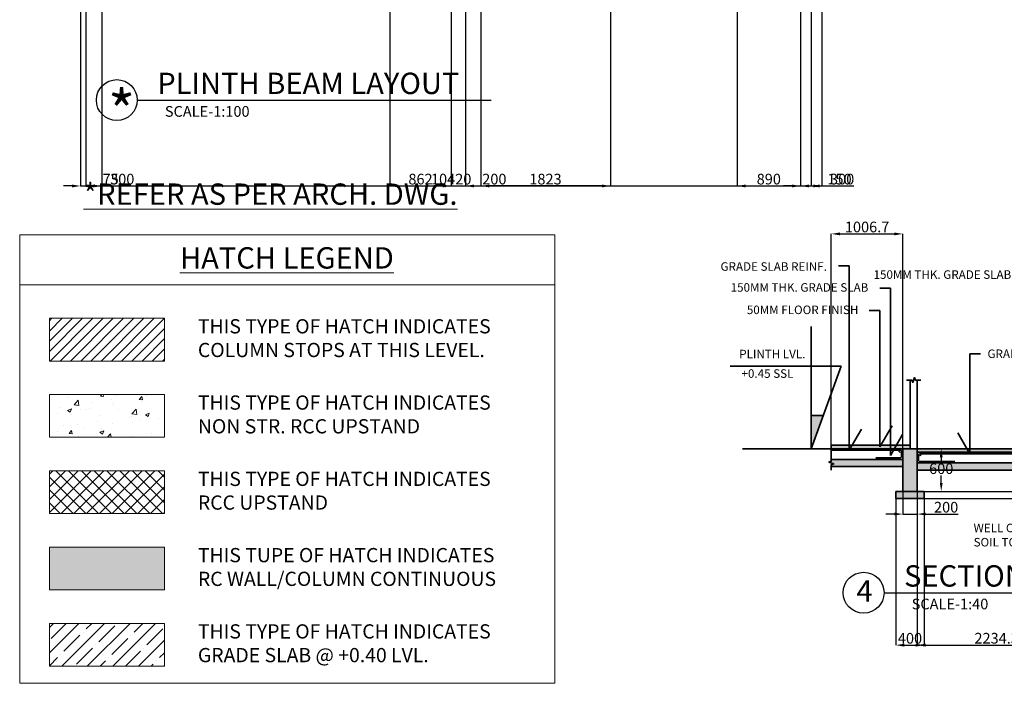
# Model space of a CAD drawing. Units: millimetres. Extents: x -174 to 32373, y 27344 to 53129.
# Tile 2 of 7: x 7596 to 21438, y 27344 to 36674. Entities that reach past the tile are written whole.
import ezdxf

# ---------------------------------------------------------------- set-up
doc = ezdxf.new("R2010")
doc.units = ezdxf.units.MM
doc.header["$LTSCALE"] = 50
for name, color, linetype, lineweight in [('S-ANNO-DIMS', 2, 'Continuous', 18), ('S-ANNO-LEGD', 7, 'Continuous', 18), ('S-ANNO-SYMB', 4, 'Continuous', 25), ('S-ANNO-TEXT', 3, 'Continuous', 18), ('S-DETL', 7, 'Continuous', 35), ('S-PATT', 8, 'Continuous', 13), ('S-REIN', 1, 'Continuous', 25)]:
    doc.layers.add(name, color=color, linetype=linetype, lineweight=lineweight)
doc.styles.get("Standard").update_dxf_attribs({"font": 'arial.ttf'})
doc.dimstyles.new('ISO-25', dxfattribs={"dimtxt": 150, "dimasz": 120, "dimexe": 1.25, "dimexo": 0.625, "dimtad": 1, "dimtih": 1, "dimtoh": 1, "dimdec": 0, "dimtxsty": 'Standard', "dimcen": 2.5, "dimadec": 0, "dimazin": 0, "dimtfac": 1, "dimtdec": 0, "dimtmove": 0, "dimatfit": 3, "dimfxl": 1, "dimarcsym": 0})

# ---------------------------------------------------------------- blocks, each defined once
blk = doc.blocks.new('*D26')
at = {"layer": 'Defpoints', "color": 0, "transparency": 16777216}
for p in [(20012, 30042), (20212, 30042), (20212, 29723)]:
    blk.add_point(p, dxfattribs=at)
at = {"layer": 'S-ANNO-DIMS', "color": 0, "lineweight": -2, "transparency": 16777216}
for p, q in [((20012, 30041), (20012, 29722)), ((20212, 30041), (20212, 29722)), ((19892, 29723), (19772, 29723)), ((20012, 29723), (20212, 29723)), ((20332, 29723), (20787, 29723))]:
    blk.add_line(p, q, dxfattribs=at)
at = {"layer": 'S-ANNO-DIMS', "color": 0, "transparency": 16777216}
for points in [[(19892, 29743), (19892, 29703), (20012, 29723)], [(20332, 29743), (20332, 29703), (20212, 29723)]]:
    blk.add_solid(points, dxfattribs=at)
at = {"layer": 'S-ANNO-DIMS', "color": 0, "transparency": 16777216, "insert": (20620, 29800), "char_height": 150, "attachment_point": 5}
blk.add_mtext('200', dxfattribs=at)
blk = doc.blocks.new('*D28')
at = {"layer": 'Defpoints', "color": 0, "transparency": 16777216}
for p in [(20212, 30642), (20212, 30042), (20551, 30042)]:
    blk.add_point(p, dxfattribs=at)
at = {"layer": 'S-ANNO-DIMS', "color": 0, "lineweight": -2, "transparency": 16777216}
for p, q in [((20213, 30642), (20552, 30642)), ((20551, 30522), (20551, 30419)), ((20551, 30162), (20551, 30265)), ((20213, 30042), (20552, 30042))]:
    blk.add_line(p, q, dxfattribs=at)
at = {"layer": 'S-ANNO-DIMS', "color": 0, "transparency": 16777216}
for points in [[(20531, 30522), (20571, 30522), (20551, 30642)], [(20531, 30162), (20571, 30162), (20551, 30042)]]:
    blk.add_solid(points, dxfattribs=at)
at = {"layer": 'S-ANNO-DIMS', "color": 0, "transparency": 16777216, "insert": (20551, 30342), "char_height": 150, "attachment_point": 5}
blk.add_mtext('600', dxfattribs=at)
blk = doc.blocks.new('SECTION-MARK')
blk.add_line((575, 287), (4248, 287))
blk.add_circle((287, 287), 287)
blk = doc.blocks.new('*D36')
at = {"layer": 'Defpoints', "color": 0, "transparency": 16777216}
for p in [(8452, 38444), (18872, 38369), (18872, 34336)]:
    blk.add_point(p, dxfattribs=at)
at = {"layer": 'S-ANNO-DIMS', "color": 0, "lineweight": -2, "transparency": 16777216}
for p, q in [((8452, 38443), (8452, 34335)), ((18872, 38368), (18872, 34335)), ((8572, 34336), (18752, 34336))]:
    blk.add_line(p, q, dxfattribs=at)
at = {"layer": 'S-ANNO-DIMS', "color": 0, "transparency": 16777216}
for points in [[(8572, 34356), (8572, 34316), (8452, 34336)], [(18752, 34356), (18752, 34316), (18872, 34336)]]:
    blk.add_solid(points, dxfattribs=at)
at = {"layer": 'S-ANNO-DIMS', "color": 0, "transparency": 16777216, "insert": (13662, 34413), "char_height": 150, "attachment_point": 5}
blk.add_mtext('10420', dxfattribs=at)
blk = doc.blocks.new('*D37')
at = {"layer": 'Defpoints', "color": 0, "transparency": 16777216}
for p in [(8452, 38444), (8527, 36932), (8527, 34336)]:
    blk.add_point(p, dxfattribs=at)
at = {"layer": 'S-ANNO-DIMS', "color": 0, "lineweight": -2, "transparency": 16777216}
for p, q in [((8452, 38443), (8452, 34335)), ((8527, 36931), (8527, 34335)), ((8332, 34336), (8212, 34336)), ((8452, 34336), (8527, 34336)), ((8647, 34336), (8983, 34336))]:
    blk.add_line(p, q, dxfattribs=at)
at = {"layer": 'S-ANNO-DIMS', "color": 0, "transparency": 16777216}
for points in [[(8332, 34356), (8332, 34316), (8452, 34336)], [(8647, 34356), (8647, 34316), (8527, 34336)]]:
    blk.add_solid(points, dxfattribs=at)
at = {"layer": 'S-ANNO-DIMS', "color": 0, "transparency": 16777216, "insert": (8875, 34413), "char_height": 150, "attachment_point": 5}
blk.add_mtext('75', dxfattribs=at)
blk = doc.blocks.new('*D38')
at = {"layer": 'Defpoints', "color": 0, "transparency": 16777216}
for p in [(18572, 38369), (18722, 36932), (18722, 34336)]:
    blk.add_point(p, dxfattribs=at)
at = {"layer": 'S-ANNO-DIMS', "color": 0, "lineweight": -2, "transparency": 16777216}
for p, q in [((18572, 38368), (18572, 34335)), ((18722, 36931), (18722, 34335)), ((18452, 34336), (18332, 34336)), ((18572, 34336), (18722, 34336)), ((18842, 34336), (19280, 34336))]:
    blk.add_line(p, q, dxfattribs=at)
at = {"layer": 'S-ANNO-DIMS', "color": 0, "transparency": 16777216}
for points in [[(18452, 34356), (18452, 34316), (18572, 34336)], [(18842, 34356), (18842, 34316), (18722, 34336)]]:
    blk.add_solid(points, dxfattribs=at)
at = {"layer": 'S-ANNO-DIMS', "color": 0, "transparency": 16777216, "insert": (19121, 34413), "char_height": 150, "attachment_point": 5}
blk.add_mtext('150', dxfattribs=at)
blk = doc.blocks.new('*D41')
at = {"layer": 'Defpoints', "color": 0, "transparency": 16777216}
for p in [(8452, 38444), (8752, 38444), (8752, 34336)]:
    blk.add_point(p, dxfattribs=at)
at = {"layer": 'S-ANNO-DIMS', "color": 0, "lineweight": -2, "transparency": 16777216}
for p, q in [((8452, 38443), (8452, 34335)), ((8752, 38443), (8752, 34335)), ((8572, 34336), (8632, 34336)), ((8752, 34336), (9204, 34336))]:
    blk.add_line(p, q, dxfattribs=at)
at = {"layer": 'S-ANNO-DIMS', "color": 0, "transparency": 16777216}
for points in [[(8572, 34356), (8572, 34316), (8452, 34336)], [(8632, 34356), (8632, 34316), (8752, 34336)]]:
    blk.add_solid(points, dxfattribs=at)
at = {"layer": 'S-ANNO-DIMS', "color": 0, "transparency": 16777216, "insert": (9038, 34413), "char_height": 150, "attachment_point": 5}
blk.add_mtext('300', dxfattribs=at)
blk = doc.blocks.new('*D44')
at = {"layer": 'Defpoints', "color": 0, "transparency": 16777216}
for p in [(13662, 45234), (13862, 45234), (13862, 34336)]:
    blk.add_point(p, dxfattribs=at)
at = {"layer": 'S-ANNO-DIMS', "color": 0, "lineweight": -2, "transparency": 16777216}
for p, q in [((13662, 45233), (13662, 34335)), ((13862, 45233), (13862, 34335)), ((13542, 34336), (13422, 34336)), ((13662, 34336), (13862, 34336)), ((13982, 34336), (14436, 34336))]:
    blk.add_line(p, q, dxfattribs=at)
at = {"layer": 'S-ANNO-DIMS', "color": 0, "transparency": 16777216}
for points in [[(13542, 34356), (13542, 34316), (13662, 34336)], [(13982, 34356), (13982, 34316), (13862, 34336)]]:
    blk.add_solid(points, dxfattribs=at)
at = {"layer": 'S-ANNO-DIMS', "color": 0, "transparency": 16777216, "insert": (14269, 34413), "char_height": 150, "attachment_point": 5}
blk.add_mtext('200', dxfattribs=at)
blk = doc.blocks.new('*D46')
at = {"layer": 'Defpoints', "color": 0, "transparency": 16777216}
for p in [(18572, 38369), (18872, 38369), (18872, 34336)]:
    blk.add_point(p, dxfattribs=at)
at = {"layer": 'S-ANNO-DIMS', "color": 0, "lineweight": -2, "transparency": 16777216}
for p, q in [((18572, 38368), (18572, 34335)), ((18872, 38368), (18872, 34335)), ((18692, 34336), (18752, 34336)), ((18872, 34336), (19324, 34336))]:
    blk.add_line(p, q, dxfattribs=at)
at = {"layer": 'S-ANNO-DIMS', "color": 0, "transparency": 16777216}
for points in [[(18692, 34356), (18692, 34316), (18572, 34336)], [(18752, 34356), (18752, 34316), (18872, 34336)]]:
    blk.add_solid(points, dxfattribs=at)
at = {"layer": 'S-ANNO-DIMS', "color": 0, "transparency": 16777216, "insert": (19158, 34413), "char_height": 150, "attachment_point": 5}
blk.add_mtext('300', dxfattribs=at)
blk = doc.blocks.new('*D48')
at = {"layer": 'Defpoints', "color": 0, "transparency": 16777216}
for p in [(17682, 43024), (18572, 38669), (18572, 34336)]:
    blk.add_point(p, dxfattribs=at)
at = {"layer": 'S-ANNO-DIMS', "color": 0, "lineweight": -2, "transparency": 16777216}
for p, q in [((17682, 43023), (17682, 34335)), ((18572, 38668), (18572, 34335)), ((17802, 34336), (18452, 34336))]:
    blk.add_line(p, q, dxfattribs=at)
at = {"layer": 'S-ANNO-DIMS', "color": 0, "transparency": 16777216}
for points in [[(17802, 34356), (17802, 34316), (17682, 34336)], [(18452, 34356), (18452, 34316), (18572, 34336)]]:
    blk.add_solid(points, dxfattribs=at)
at = {"layer": 'S-ANNO-DIMS', "color": 0, "transparency": 16777216, "insert": (18127, 34413), "char_height": 150, "attachment_point": 5}
blk.add_mtext('890', dxfattribs=at)
blk = doc.blocks.new('*D58')
at = {"layer": 'Defpoints', "color": 0, "transparency": 16777216}
for p in [(15900, 43174), (14077, 43024), (14077, 34336)]:
    blk.add_point(p, dxfattribs=at)
at = {"layer": 'S-ANNO-DIMS', "color": 0, "lineweight": -2, "transparency": 16777216}
for p, q in [((15900, 43173), (15900, 34335)), ((14077, 43023), (14077, 34335)), ((15780, 34336), (14197, 34336))]:
    blk.add_line(p, q, dxfattribs=at)
at = {"layer": 'S-ANNO-DIMS', "color": 0, "transparency": 16777216}
for points in [[(14197, 34356), (14197, 34316), (14077, 34336)], [(15780, 34356), (15780, 34316), (15900, 34336)]]:
    blk.add_solid(points, dxfattribs=at)
at = {"layer": 'S-ANNO-DIMS', "color": 0, "transparency": 16777216, "insert": (14988, 34413), "char_height": 150, "attachment_point": 5}
blk.add_mtext('1823', dxfattribs=at)
blk = doc.blocks.new('*D59')
at = {"layer": 'Defpoints', "color": 0, "transparency": 16777216}
for p in [(12800, 46609), (13662, 46609), (13662, 34336)]:
    blk.add_point(p, dxfattribs=at)
at = {"layer": 'S-ANNO-DIMS', "color": 0, "lineweight": -2, "transparency": 16777216}
for p, q in [((12800, 46608), (12800, 34335)), ((13662, 46608), (13662, 34335)), ((12920, 34336), (13542, 34336))]:
    blk.add_line(p, q, dxfattribs=at)
at = {"layer": 'S-ANNO-DIMS', "color": 0, "transparency": 16777216}
for points in [[(12920, 34356), (12920, 34316), (12800, 34336)], [(13542, 34356), (13542, 34316), (13662, 34336)]]:
    blk.add_solid(points, dxfattribs=at)
at = {"layer": 'S-ANNO-DIMS', "color": 0, "transparency": 16777216, "insert": (13231, 34413), "char_height": 150, "attachment_point": 5}
blk.add_mtext('862', dxfattribs=at)
blk = doc.blocks.new('*D85')
at = {"layer": 'Defpoints', "color": 0, "transparency": 16777216}
for p in [(20212, 30042), (22447, 30042), (22447, 27880)]:
    blk.add_point(p, dxfattribs=at)
at = {"layer": 'S-ANNO-DIMS', "color": 0, "lineweight": -2, "transparency": 16777216}
for p, q in [((20212, 30041), (20212, 27879)), ((22447, 30041), (22447, 27879)), ((20332, 27880), (22327, 27880))]:
    blk.add_line(p, q, dxfattribs=at)
at = {"layer": 'S-ANNO-DIMS', "color": 0, "transparency": 16777216}
for points in [[(20332, 27900), (20332, 27860), (20212, 27880)], [(22327, 27900), (22327, 27860), (22447, 27880)]]:
    blk.add_solid(points, dxfattribs=at)
at = {"layer": 'S-ANNO-DIMS', "color": 0, "transparency": 16777216, "insert": (21330, 27958), "char_height": 150, "attachment_point": 5}
blk.add_mtext('2234.3', dxfattribs=at)
blk = doc.blocks.new('*D89')
at = {"layer": 'Defpoints', "color": 0, "transparency": 16777216}
for p in [(20012, 33662), (19006, 30692), (20012, 30642)]:
    blk.add_point(p, dxfattribs=at)
at = {"layer": 'S-ANNO-DIMS', "color": 0, "lineweight": -2, "transparency": 16777216}
for p, q in [((19006, 30692), (19006, 33664)), ((19126, 33662), (19892, 33662)), ((20012, 30642), (20012, 33664))]:
    blk.add_line(p, q, dxfattribs=at)
at = {"layer": 'S-ANNO-DIMS', "color": 0, "transparency": 16777216}
for points in [[(19126, 33682), (19126, 33642), (19006, 33662)], [(19892, 33682), (19892, 33642), (20012, 33662)]]:
    blk.add_solid(points, dxfattribs=at)
at = {"layer": 'S-ANNO-DIMS', "color": 0, "transparency": 16777216, "insert": (19509, 33740), "char_height": 150, "attachment_point": 5}
blk.add_mtext('1006.7', dxfattribs=at)
blk = doc.blocks.new('*D91')
at = {"layer": 'Defpoints', "color": 0, "transparency": 16777216}
for p in [(19912, 29942), (20312, 29942), (20312, 27880)]:
    blk.add_point(p, dxfattribs=at)
at = {"layer": 'S-ANNO-DIMS', "color": 0, "lineweight": -2, "transparency": 16777216}
for p, q in [((19912, 29941), (19912, 27879)), ((20312, 29941), (20312, 27879)), ((20032, 27880), (20192, 27880))]:
    blk.add_line(p, q, dxfattribs=at)
at = {"layer": 'S-ANNO-DIMS', "color": 0, "transparency": 16777216}
for points in [[(20032, 27900), (20032, 27860), (19912, 27880)], [(20192, 27900), (20192, 27860), (20312, 27880)]]:
    blk.add_solid(points, dxfattribs=at)
at = {"layer": 'S-ANNO-DIMS', "color": 0, "transparency": 16777216, "insert": (20112, 27957), "char_height": 150, "attachment_point": 5}
blk.add_mtext('400', dxfattribs=at)
blk = doc.blocks.new('*D92')
at = {"layer": 'Defpoints', "color": 0, "transparency": 16777216}
for p in [(20312, 30042), (24149, 30042), (20312, 29942)]:
    blk.add_point(p, dxfattribs=at)
at = {"layer": 'S-ANNO-DIMS', "color": 0, "lineweight": -2, "transparency": 16777216}
for p, q in [((24149, 30162), (24149, 30282)), ((24149, 30282), (24466, 30282)), ((20313, 30042), (24150, 30042)), ((24149, 29942), (24149, 30042)), ((20313, 29942), (24150, 29942)), ((24149, 29822), (24149, 29702))]:
    blk.add_line(p, q, dxfattribs=at)
at = {"layer": 'S-ANNO-DIMS', "color": 0, "transparency": 16777216}
for points in [[(24129, 30162), (24169, 30162), (24149, 30042)], [(24129, 29822), (24169, 29822), (24149, 29942)]]:
    blk.add_solid(points, dxfattribs=at)
at = {"layer": 'S-ANNO-DIMS', "color": 0, "transparency": 16777216, "insert": (24308, 30359), "char_height": 150, "attachment_point": 5}
blk.add_mtext('100', dxfattribs=at)

msp = doc.modelspace()

# ---------------------------------------------------------------- hatches: boundary and pattern name
at = {"layer": 'S-ANNO-SYMB'}
h = msp.add_hatch(color=256, dxfattribs=at)
h.dxf.hatch_style = 1
h.paths.add_polyline_path([(18722.49, 30641.75), (18891.71, 31106.67), (18722.49, 31106.67)])
at = {"layer": 'S-PATT'}
h = msp.add_hatch(dxfattribs=at)
h.set_pattern_fill('ANSI31', color=256, scale=32)
h.paths.add_polyline_path([(9631.43, 32476.32), (8014.28, 32476.32), (8014.28, 31874.81), (9631.43, 31874.81)])
h = msp.add_hatch(dxfattribs=at)
h.set_pattern_fill('AR-CONC', color=256, scale=3)
h.paths.add_polyline_path([(9631.43, 31403.9), (8014.28, 31403.9), (8014.28, 30802.39), (9631.43, 30802.39)])
h = msp.add_hatch(dxfattribs=at)
h.set_pattern_fill('ANGLE', color=256, scale=5)
h.set_pattern_definition([(0, (-5178.336, 733.413), (0, 34.925), [25.4, -9.525]), (90, (-5178.336, 733.413), (-34.925, 2e-15), [25.4, -9.525])])
h.paths.add_polyline_path([(22446.68, 30591.75), (22446.68, 30641.75), (20212.39, 30641.75), (20212.39, 30591.75)])
h.paths.add_polyline_path([(20012.39, 30641.75), (20112.39, 30641.75), (20112.39, 30691.75), (19005.68, 30691.75), (19005.68, 30641.75)])
h.paths.add_polyline_path([(22546.68, 30691.75), (22546.68, 30641.75), (22646.68, 30641.75), (23664.24, 30641.75), (23664.24, 30691.75)])
h = msp.add_hatch(color=256, dxfattribs=at)
h.dxf.hatch_style = 1
h.paths.add_polyline_path([(20212.39, 30641.75), (20012.39, 30641.75), (20012.39, 30041.75), (20212.39, 30041.75)])
h.paths.add_polyline_path([(22646.68, 30641.75), (22446.68, 30641.75), (22446.68, 30041.75), (22646.68, 30041.75)])
h = msp.add_hatch(dxfattribs=at)
h.set_pattern_fill('AR-CONC', color=256)
h.set_pattern_definition([(50, (-5178.34, 733.41), (182.18467, -15.9391), [19.05, -209.55]), (355, (-5178.34, 733.41), (-35.2434, 191.05685), [15.24, -167.6406]), (100.45144, (-5163.15, 732.09), (146.94125, 175.11775), [16.19, -178.09024]), (46.1842, (-5178.34, 784.21), (271.079, -42.0423), [28.575, -314.325]), (96.63556, (-5155.75, 780.7), (237.4041, 247.4261), [24.285, -267.1356]), (351.18415, (-5178.34, 784.2), (237.4041, 247.4261), [22.86, -251.4597]), (21, (-5152.94, 771.51), (151.6144, -102.2652), [19.05, -209.55]), (326, (-5152.94, 771.51), (61.802, 184.188), [15.24, -167.64]), (71.45144, (-5140.3, 762.99), (213.4164, 81.9228), [16.19, -178.0899]), (37.5, (-5178.336, 733.413), (3.0886, 84.55504), [0, -165.608, 0, -170.18, 0, -168.275]), (7.5, (-5178.34, 733.41), (66.81966, 100.18057), [0, -97.028, 0, -161.798, 0, -64.135]), (327.5, (-5234.98, 733.41), (135.5906, -5.72874), [0, -63.5, 0, -198.12, 0, -262.89]), (317.5, (-5260.38, 733.41), (148.12918, 25.4265), [0, -82.55, 0, -131.572, 0, -186.69])])
h.paths.add_polyline_path([(20312.39, 29941.75), (20312.39, 30041.75), (20212.39, 30041.75), (20012.39, 30041.75), (19912.39, 30041.75), (19912.39, 29941.75)])
h.paths.add_polyline_path([(22746.68, 29941.75), (22746.68, 30041.75), (22646.68, 30041.75), (22446.68, 30041.75), (22346.68, 30041.75), (22346.68, 29941.75)])
h.paths.add_polyline_path([(22446.68, 30341.75), (22446.68, 30441.75), (20212.39, 30441.75), (20212.39, 30341.75)])
h.paths.add_polyline_path([(23664.24, 30391.75), (23664.24, 30441.75), (23629.9, 30454.25), (23664.24, 30466.75), (23664.24, 30491.75), (22646.68, 30491.75), (22646.68, 30391.75)])
h.paths.add_polyline_path([(20012.39, 30391.75), (20012.39, 30491.75), (19005.68, 30491.75), (19005.68, 30441.75), (19040.02, 30429.25), (19005.68, 30416.75), (19005.68, 30391.75)])
h = msp.add_hatch(dxfattribs=at)
h.set_pattern_fill('ANSI37', color=256, scale=40)
h.paths.add_polyline_path([(9631.43, 30331.48), (8014.28, 30331.48), (8014.28, 29729.97), (9631.43, 29729.97)])
h = msp.add_hatch(color=256, dxfattribs=at)
h.dxf.hatch_style = 1
h.paths.add_polyline_path([(9631.43, 29259.07), (8014.28, 29259.07), (8014.28, 28657.56), (9631.43, 28657.56)])
h = msp.add_hatch(dxfattribs=at)
h.set_pattern_fill('ANSI35', color=256, scale=40)
h.paths.add_polyline_path([(9631.43, 28186.65), (8014.28, 28186.65), (8014.28, 27585.14), (9631.43, 27585.14)])

# ---------------------------------------------------------------- linework, layer by layer
at = {"layer": 'S-ANNO-LEGD'}
for p, q in [((7596.47, 33647.22), (15117.8, 33647.22)), ((7596.47, 27343.65), (7596.47, 33647.22)), ((15117.8, 33647.22), (15117.8, 27343.65)), ((7596.47, 32947.22), (15117.8, 32947.22)), ((15117.8, 27343.65), (7596.47, 27343.65))]:
    msp.add_line(p, q, dxfattribs=at)
for points in [[(8014.28, 32476.32), (9631.43, 32476.32), (9631.43, 31874.81), (8014.28, 31874.81)], [(8014.28, 31403.9), (9631.43, 31403.9), (9631.43, 30802.39), (8014.28, 30802.39)], [(8014.28, 30331.48), (9631.43, 30331.48), (9631.43, 29729.97), (8014.28, 29729.97)], [(8014.28, 29259.07), (9631.43, 29259.07), (9631.43, 28657.56), (8014.28, 28657.56)], [(8014.28, 28186.65), (9631.43, 28186.65), (9631.43, 27585.14), (8014.28, 27585.14)]]:
    msp.add_lwpolyline(points, close=True, dxfattribs=at)
at = {"layer": 'S-ANNO-SYMB'}
msp.add_line((9249.08, 35543.22), (14224.21, 35543.22), dxfattribs=at)
msp.add_circle((8961.62, 35543.22), 287.47, dxfattribs=at)
at = {"layer": 'S-DETL'}
for p, q in [((19258.94, 33212.37), (19108.63, 33212.37)), ((19258.94, 30621.75), (19258.94, 33212.37)), ((19836.67, 32901), (19686.35, 32901)), ((19836.67, 30548.08), (19836.67, 32901)), ((19689.54, 32585.77), (19539.22, 32585.77)), ((19689.54, 30667.42), (19689.54, 32585.77)), ((18722.49, 30641.75), (18722.49, 32360.55)), ((20953.23, 30571.75), (20953.23, 31975.83)), ((20953.23, 31975.83), (21105.39, 31975.83)), ((19145.31, 31803.43), (17586.18, 31803.43)), ((18722.49, 30641.75), (19145.31, 31803.43)), ((20112.39, 30641.75), (20112.39, 31607.24)), ((20212.39, 30641.75), (20212.39, 31607.24)), ((18722.49, 31106.67), (18891.71, 31106.67)), ((19258.94, 30621.75), (19428.95, 30916.22)), ((19689.54, 30667.42), (19859.55, 30961.89)), ((20953.23, 30571.75), (20783.22, 30866.22)), ((19836.67, 30548.08), (20006.68, 30842.55)), ((20012.39, 30641.75), (17756.66, 30641.75)), ((20112.39, 30691.75), (19005.68, 30691.75)), ((19005.68, 30691.75), (19005.68, 30491.75)), ((19976.39, 30621.75), (19005.68, 30621.75)), ((19992.39, 30605.75), (19992.39, 30527.75)), ((20212.39, 30641.75), (20012.39, 30641.75)), ((20012.39, 30641.75), (20012.39, 30041.75)), ((20112.39, 30641.75), (20112.39, 30691.75)), ((20212.39, 30641.75), (22446.68, 30641.75)), ((20212.39, 30041.75), (20212.39, 30641.75)), ((20212.39, 30591.75), (22446.68, 30591.75)), ((20012.39, 30491.75), (19005.68, 30491.75)), ((19976.39, 30511.75), (19630.72, 30511.75)), ((20232.39, 30477.75), (20232.39, 30555.75)), ((20248.39, 30571.75), (22410.68, 30571.75)), ((20248.39, 30461.75), (20740.54, 30461.75)), ((20012.39, 30391.75), (19005.68, 30391.75)), ((20212.39, 30441.75), (22446.68, 30441.75)), ((20212.39, 30341.75), (22446.68, 30341.75)), ((19912.39, 29941.75), (19912.39, 30041.75)), ((19912.39, 30041.75), (20012.39, 30041.75)), ((20012.39, 30041.75), (20212.39, 30041.75)), ((20212.39, 30041.75), (20312.39, 30041.75)), ((20312.39, 30041.75), (20312.39, 29941.75)), ((20312.39, 29941.75), (19912.39, 29941.75))]:
    msp.add_line(p, q, dxfattribs=at)
for points in [[(20062.39, 31607.24), (20137.39, 31607.24), (20149.89, 31572.9), (20174.89, 31641.59), (20187.39, 31607.24), (20262.39, 31607.24)], [(19005.68, 30541.75), (19005.68, 30466.75), (18971.33, 30454.25), (19040.02, 30429.25), (19005.68, 30416.75), (19005.68, 30341.75)]]:
    msp.add_lwpolyline(points, dxfattribs=at)
at = {"layer": 'S-REIN'}
for centre in [(19976.39, 30605.75), (20248.39, 30555.75)]:
    msp.add_circle(centre, 16, dxfattribs=at)
for centre, start, end in [((19976.39, 30605.75), 0, 90), ((19976.39, 30527.75), 270, 0), ((20248.39, 30555.75), 90, 180), ((20248.39, 30477.75), 180, 270)]:
    msp.add_arc(centre, 16, start, end, dxfattribs=at)

# ---------------------------------------------------------------- block references
at = {"layer": 'S-ANNO-SYMB'}
msp.add_blockref('SECTION-MARK', (19172.63, 28330.26), dxfattribs=at)

# ---------------------------------------------------------------- texts
at = {"layer": 'S-ANNO-TEXT', "attachment_point": 1}
for s, width, insert, char_height in [('PLINTH BEAM LAYOUT', 6501.8432, (9530.62, 35928.76), 300), ('*', 6501.8432, (8837.6, 35677), 600), ('SCALE-1:100', 1913.0414, (9637.43, 35459.15), 150), ('{\\L*REFER AS PER ARCH. DWG.}', 6501.8432, (8493.88, 34370.99), 300), ('{\\LHATCH LEGEND}', 5016.1493, (9849.36, 33474.61), 300), ('GRADE SLAB REINF.', 1913.0414, (17448.78, 33263.42), 120), ('150MM THK. GRADE SLAB', 2289.8517, (19599.45, 33150.3), 120), ('150MM THK. GRADE SLAB', 2289.8517, (17590.5, 32969.37), 120), ('50MM FLOOR FINISH', 2289.8517, (17818.33, 32654.51), 120), ('THIS TYPE OF HATCH INDICATES\\PCOLUMN STOPS AT THIS LEVEL.', 5016.1493, (10101.65, 32463.14), 200), ('PLINTH LVL.', 1913.0414, (17711.58, 32032.68), 120), ('GRADE SLAB REINF.', 2900.7274, (21201.77, 32036.94), 120), ('+0.45 SSL', 1913.0414, (17743.26, 31758.71), 120), ('THIS TYPE OF HATCH INDICATES\\PNON STR. RCC UPSTAND', 5016.1493, (10101.65, 31390.72), 200), ('THIS TYPE OF HATCH INDICATES\\PRCC UPSTAND', 5016.1493, (10101.65, 30318.3), 200), ('WELL COMPACTED\\PSOIL TO 95% MDD.', 1913.0414, (21006, 29587.7), 120), ('THIS TUPE OF HATCH INDICATES \\PRC WALL/COLUMN CONTINUOUS', 5016.1493, (10101.65, 29245.89), 200), ('SECTION 04-04', 6501.8432, (20029.1, 29003.27), 300), ('4', 6501.8432, (19359.54, 28793.09), 300), ('SCALE-1:40', 1913.0414, (20135.91, 28533.66), 150), ('THIS TYPE OF HATCH INDICATES\\PGRADE SLAB @ +0.40 LVL.', 5016.1493, (10101.65, 28173.47), 200)]:
    msp.add_mtext_dynamic_manual_height_columns(s, width=width, gutter_width=12.5, heights=[0], dxfattribs=dict(at, insert=insert, char_height=char_height))

# ---------------------------------------------------------------- dimensions: what is measured, and where the dimension line sits
at = {"layer": 'S-ANNO-DIMS'}
for base, p1, p2, override, picture, middle in [((13661.66, 34335.75), (12799.66, 46608.76), (13661.66, 46608.76), {"dimdec": 0, "dimlfac": 1, "dimrnd": 0, "dimzin": 0, "dimdsep": 46, "dimlunit": 2}, '*D59', (13230.66, 34412.96)), ((13861.66, 34335.75), (13661.66, 45233.76), (13861.66, 45233.76), {"dimdec": 0, "dimlfac": 1, "dimrnd": 0, "dimzin": 0, "dimdsep": 46, "dimlunit": 2}, '*D44', (14269.02, 34412.96)), ((14076.66, 34335.75), (15899.72, 43173.76), (14076.66, 43023.76), {"dimdec": 0, "dimlfac": 1, "dimrnd": 0, "dimzin": 0, "dimdsep": 46, "dimlunit": 2}, '*D58', (14988.19, 34413.01)), ((18571.66, 34335.75), (17681.66, 43023.76), (18571.66, 38668.76), {"dimdec": 0, "dimlfac": 1, "dimrnd": 0, "dimzin": 0, "dimdsep": 46, "dimlunit": 2}, '*D48', (18126.66, 34412.96)), ((8526.66, 34335.75), (8451.66, 38443.76), (8526.66, 36931.64), {"dimdec": 0, "dimlfac": 1, "dimrnd": 0, "dimzin": 0, "dimdsep": 46, "dimlunit": 2}, '*D37', (8874.67, 34412.65)), ((18871.66, 34335.75), (8451.66, 38443.76), (18871.66, 38368.76), {"dimdec": 0, "dimlfac": 1, "dimrnd": 0, "dimzin": 0, "dimdsep": 46, "dimlunit": 2}, '*D36', (13661.66, 34412.96)), ((8751.66, 34335.75), (8451.66, 38443.76), (8751.66, 38443.76), {"dimdec": 0, "dimlfac": 1, "dimrnd": 0, "dimzin": 0, "dimdsep": 46, "dimlunit": 2}, '*D41', (9037.69, 34413.01)), ((18721.66, 34335.75), (18571.66, 38368.76), (18721.66, 36931.64), {"dimdec": 0, "dimlfac": 1, "dimrnd": 0, "dimzin": 0, "dimdsep": 46, "dimlunit": 2}, '*D38', (19120.68, 34412.96)), ((18871.66, 34335.75), (18571.66, 38368.76), (18871.66, 38368.76), {"dimdec": 0, "dimlfac": 1, "dimrnd": 0, "dimzin": 0, "dimdsep": 46, "dimlunit": 2}, '*D46', (19157.69, 34413.01)), ((20012.39, 33662.37), (19005.68, 30691.75), (20012.39, 30641.75), {"dimdec": 1, "dimlfac": 1, "dimrnd": 0, "dimzin": 0, "dimdsep": 46, "dimlunit": 2}, '*D89', (19509.03, 33739.58)), ((20212.39, 29722.95), (20012.39, 30041.75), (20212.39, 30041.75), {"dimclrd": 0, "dimclre": 0, "dimclrt": 0}, '*D26', (20619.75, 29800.17)), ((22446.68, 27880.26), (20212.39, 30041.75), (22446.68, 30041.75), {"dimdec": 1, "dimlfac": 1, "dimrnd": 0, "dimzin": 0, "dimdsep": 46, "dimlunit": 2}, '*D85', (21329.54, 27957.52)), ((20312.39, 27880.26), (19912.39, 29941.75), (20312.39, 29941.75), {"dimdec": 0, "dimlfac": 1, "dimrnd": 0, "dimzin": 0, "dimdsep": 46, "dimlunit": 2}, '*D91', (20112.39, 27957.47))]:
    dim = msp.add_linear_dim(base=base, p1=p1, p2=p2, dimstyle='ISO-25', override=override, dxfattribs=at)
    dim.commit()
    dim.dimension.update_dxf_attribs({"geometry": picture, "text_midpoint": middle})
for base, p1, p2, override, picture, middle in [((20550.7, 30041.75), (20212.39, 30641.75), (20212.39, 30041.75), {"dimclrd": 0, "dimclre": 0, "dimclrt": 0}, '*D28', (20550.7, 30341.75)), ((24148.59, 30041.75), (20312.39, 29941.75), (20312.39, 30041.75), {"dimdec": 0, "dimlfac": 1, "dimrnd": 0, "dimzin": 0, "dimdsep": 46, "dimlunit": 2}, '*D92', (24307.6, 30358.96))]:
    dim = msp.add_linear_dim(base=base, p1=p1, p2=p2, angle=90, dimstyle='ISO-25', override=override, dxfattribs=at)
    dim.commit()
    dim.dimension.update_dxf_attribs({"geometry": picture, "text_midpoint": middle})

doc.saveas('drawing.dxf')
